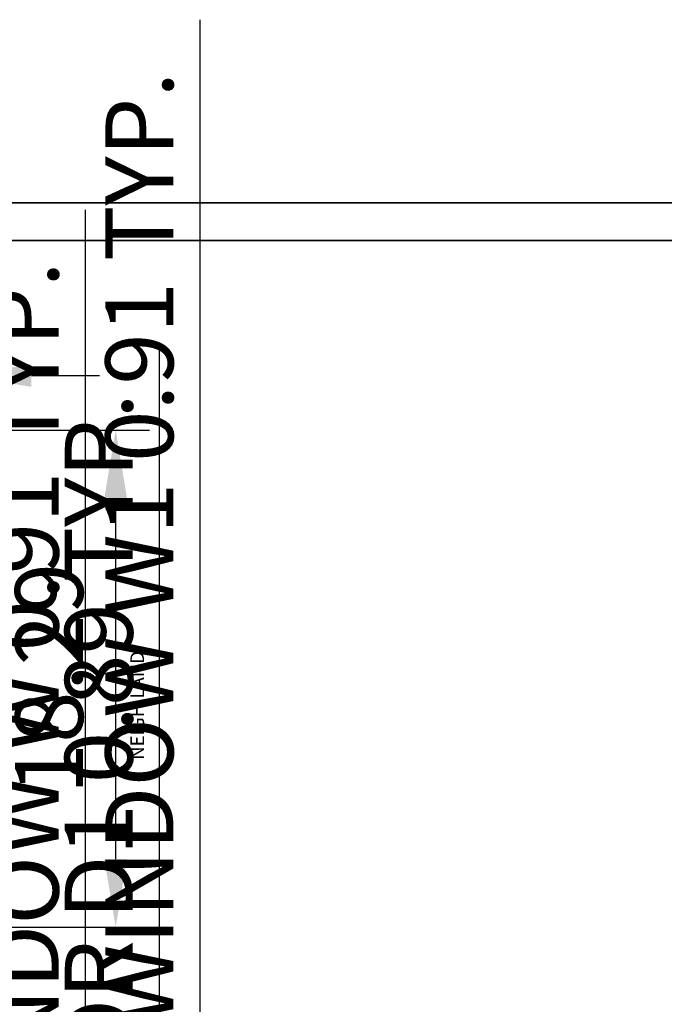
# Model space of a CAD drawing. Units: metres. Extents: x 782 to 1487, y 1262 to 7446.
# Tile 24 of 25: x 826 to 850, y 1313 to 1350. Entities that reach past the tile are written whole.
import ezdxf

# ---------------------------------------------------------------- set-up
doc = ezdxf.new("R2010")
doc.units = ezdxf.units.M
for name, color, linetype, lineweight in [('A-ANNO-DIMS', 2, 'Continuous', 18), ('A-ANNO-TEXT', 3, 'Continuous', 18), ('A-ANNO-TTLB', 7, 'Continuous', 35)]:
    doc.layers.add(name, color=color, linetype=linetype, lineweight=lineweight)
doc.styles.get("Standard").update_dxf_attribs({"font": 'arial.ttf'})
doc.dimstyles.new('ISO-25', dxfattribs={"dimtxt": 2.5, "dimasz": 2.5, "dimexe": 1.25, "dimexo": 0.625, "dimtad": 1, "dimtxsty": 'Standard', "dimcen": 2.5, "dimadec": 0, "dimazin": 0, "dimtfac": 1, "dimtmove": 0, "dimatfit": 3, "dimfxl": 1, "dimarcsym": 0})

# ---------------------------------------------------------------- blocks, each defined once
blk = doc.blocks.new('*D11')
at = {"layer": 'A-ANNO-DIMS', "color": 0, "lineweight": -2, "transparency": 16777216}
for p, q in [((824.462, 1334.623), (830.687, 1334.623)), ((829.437, 1332.123), (829.437, 1318.837)), ((824.462, 1316.337), (830.687, 1316.337))]:
    blk.add_line(p, q, dxfattribs=at)
at = {"layer": 'A-ANNO-DIMS', "color": 0, "transparency": 16777216}
for points in [[(829.02, 1332.123), (829.854, 1332.123), (829.437, 1334.623)], [(829.02, 1318.837), (829.854, 1318.837), (829.437, 1316.337)]]:
    blk.add_solid(points, dxfattribs=at)
at = {"layer": 'Defpoints', "color": 0, "transparency": 16777216}
for p in [(823.837, 1334.623), (823.837, 1316.337), (829.437, 1316.337)]:
    blk.add_point(p, dxfattribs=at)
at = {"layer": 'A-ANNO-DIMS', "color": 0, "transparency": 16777216, "insert": (827.31, 1325.48), "char_height": 2.5, "attachment_point": 5, "rotation": 90}
blk.add_mtext('18,29', dxfattribs=at)
blk = doc.blocks.new('*D12')
at = {"layer": 'A-ANNO-DIMS', "color": 0, "lineweight": -2, "transparency": 16777216}
for p, q in [((818.357, 1335.252), (818.357, 1337.877)), ((823.837, 1335.252), (823.837, 1337.877)), ((815.857, 1336.627), (805.608, 1336.627)), ((823.837, 1336.627), (818.357, 1336.627)), ((826.337, 1336.627), (828.837, 1336.627))]:
    blk.add_line(p, q, dxfattribs=at)
at = {"layer": 'A-ANNO-DIMS', "color": 0, "transparency": 16777216}
for points in [[(815.857, 1337.044), (815.857, 1336.21), (818.357, 1336.627)], [(826.337, 1337.044), (826.337, 1336.21), (823.837, 1336.627)]]:
    blk.add_solid(points, dxfattribs=at)
at = {"layer": 'Defpoints', "color": 0, "transparency": 16777216}
for p in [(818.357, 1336.627), (818.357, 1334.627), (823.837, 1334.627)]:
    blk.add_point(p, dxfattribs=at)
at = {"layer": 'A-ANNO-DIMS', "color": 0, "transparency": 16777216, "insert": (809.482, 1338.754), "char_height": 2.5, "width": 6.51678, "attachment_point": 5}
blk.add_mtext('5,48', dxfattribs=at)
blk = doc.blocks.new('*D20')
at = {"layer": 'A-ANNO-DIMS', "color": 0, "lineweight": -2, "transparency": 16777216}
for p, q in [((831.056, 1302.088), (831.056, 1337.678)), ((831.056, 1298.698), (831.056, 1299.588)), ((831.548, 1299.588), (832.306, 1299.588)), ((831.548, 1298.698), (832.306, 1298.698)), ((831.056, 1296.198), (831.056, 1293.698))]:
    blk.add_line(p, q, dxfattribs=at)
at = {"layer": 'A-ANNO-DIMS', "color": 0, "transparency": 16777216}
for points in [[(830.64, 1302.088), (831.473, 1302.088), (831.056, 1299.588)], [(830.64, 1296.198), (831.473, 1296.198), (831.056, 1298.698)]]:
    blk.add_solid(points, dxfattribs=at)
at = {"layer": 'Defpoints', "color": 0, "transparency": 16777216}
for p in [(830.923, 1299.588), (831.056, 1299.588), (830.923, 1298.698)]:
    blk.add_point(p, dxfattribs=at)
at = {"layer": 'A-ANNO-DIMS', "color": 0, "transparency": 16777216, "insert": (829.138, 1321.133), "char_height": 2.5, "attachment_point": 5, "rotation": 90}
blk.add_mtext('DOOR D1 0.89 TYP.', dxfattribs=at)
blk = doc.blocks.new('*D26')
at = {"layer": 'A-ANNO-DIMS', "color": 0, "lineweight": -2, "transparency": 16777216}
for p, q in [((828.33, 1303.223), (828.33, 1342.718)), ((828.33, 1299.809), (828.33, 1300.723)), ((828.818, 1300.723), (829.58, 1300.723)), ((828.818, 1299.809), (829.58, 1299.809)), ((828.33, 1297.309), (828.33, 1294.809))]:
    blk.add_line(p, q, dxfattribs=at)
at = {"layer": 'A-ANNO-DIMS', "color": 0, "transparency": 16777216}
for points in [[(827.913, 1303.223), (828.747, 1303.223), (828.33, 1300.723)], [(827.913, 1297.309), (828.747, 1297.309), (828.33, 1299.809)]]:
    blk.add_solid(points, dxfattribs=at)
at = {"layer": 'Defpoints', "color": 0, "transparency": 16777216}
for p in [(828.193, 1300.723), (828.33, 1300.723), (828.193, 1299.809)]:
    blk.add_point(p, dxfattribs=at)
at = {"layer": 'A-ANNO-DIMS', "color": 0, "transparency": 16777216, "insert": (826.412, 1324.22), "char_height": 2.5, "attachment_point": 5, "rotation": 90}
blk.add_mtext('WINDOW W 0.91 TYP.', dxfattribs=at)
blk = doc.blocks.new('*D28')
at = {"layer": 'A-ANNO-DIMS', "color": 0, "lineweight": -2, "transparency": 16777216}
for p, q in [((832.55, 1308.281), (832.55, 1349.718)), ((832.55, 1304.867), (832.55, 1305.781)), ((833.038, 1305.781), (833.8, 1305.781)), ((833.038, 1304.867), (833.8, 1304.867)), ((832.55, 1302.367), (832.55, 1299.867))]:
    blk.add_line(p, q, dxfattribs=at)
at = {"layer": 'A-ANNO-DIMS', "color": 0, "transparency": 16777216}
for points in [[(832.134, 1308.281), (832.967, 1308.281), (832.55, 1305.781)], [(832.134, 1302.367), (832.967, 1302.367), (832.55, 1304.867)]]:
    blk.add_solid(points, dxfattribs=at)
at = {"layer": 'Defpoints', "color": 0, "transparency": 16777216}
for p in [(832.413, 1305.781), (832.55, 1305.781), (832.413, 1304.867)]:
    blk.add_point(p, dxfattribs=at)
at = {"layer": 'A-ANNO-DIMS', "color": 0, "transparency": 16777216, "insert": (830.632, 1330.25), "char_height": 2.5, "attachment_point": 5, "rotation": 90}
blk.add_mtext('WINDOW W1 0.91 TYP.', dxfattribs=at)

msp = doc.modelspace()

# ---------------------------------------------------------------- linework, layer by layer
at = {"layer": 'A-ANNO-TTLB'}
msp.add_line((834.8075, 1341.5907), (851.2547, 1341.5907), dxfattribs=at)
for points in [[(787.4248, 1342.9861), (880.8003, 1342.9861), (880.8003, 1263.8004), (787.4248, 1263.8004)], [(883.6865, 1262.3458), (787.4248, 1262.3458), (787.4248, 1342.9861), (883.6865, 1342.9861)], [(788.8147, 1341.5907), (880.8003, 1341.5907), (880.8003, 1263.8004), (788.8147, 1263.8004)]]:
    msp.add_lwpolyline(points, close=True, dxfattribs=at)

# ---------------------------------------------------------------- texts
at = {"layer": 'A-ANNO-TEXT', "insert": (829.98, 1322.493), "char_height": 0.5, "attachment_point": 1, "rotation": 90}
msp.add_mtext_dynamic_manual_height_columns('NEIGH.LAND', width=7.994851, gutter_width=12.5, heights=[0], dxfattribs=at)

# ---------------------------------------------------------------- dimensions: what is measured, and where the dimension line sits
at = {"layer": 'A-ANNO-DIMS'}
for base, p1, p2, text, picture, middle in [((832.5503, 1305.7809), (832.4132, 1304.8669), (832.4132, 1305.7809), 'WINDOW W1 <> TYP.', '*D28', (830.6318, 1330.2497)), ((828.3302, 1300.7228), (828.1931, 1299.8088), (828.1931, 1300.7228), 'WINDOW W <> TYP.', '*D26', (826.4117, 1324.2204)), ((831.0564, 1299.5877), (830.923, 1298.6982), (830.923, 1299.5877), 'DOOR D1 <> TYP.', '*D20', (829.138, 1321.1327))]:
    dim = msp.add_linear_dim(base=base, p1=p1, p2=p2, angle=90, text=text, dimstyle='ISO-25', override={"dimdec": 2, "dimlfac": 1, "dimrnd": 0, "dimzin": 0, "dimdsep": 46, "dimlunit": 2}, dxfattribs=at)
    dim.commit()
    dim.dimension.update_dxf_attribs({"geometry": picture, "text_midpoint": middle})
dim = msp.add_linear_dim(base=(818.357, 1336.627), p1=(823.837, 1334.627), p2=(818.357, 1334.627), dimstyle='ISO-25', override={"dimclrd": 0, "dimclre": 0, "dimclrt": 0}, dxfattribs=at)
dim.commit()
dim.dimension.update_dxf_attribs({"geometry": '*D12', "text_midpoint": (809.4825, 1338.7544)})
dim = msp.add_linear_dim(base=(829.437, 1316.337), p1=(823.8366, 1334.6231), p2=(823.8366, 1316.337), angle=90, dimstyle='ISO-25', override={"dimclrd": 0, "dimclre": 0, "dimclrt": 0}, dxfattribs=at)
dim.commit()
dim.dimension.update_dxf_attribs({"geometry": '*D11', "text_midpoint": (827.3096, 1325.48)})

doc.saveas('drawing.dxf')
